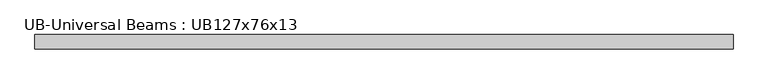
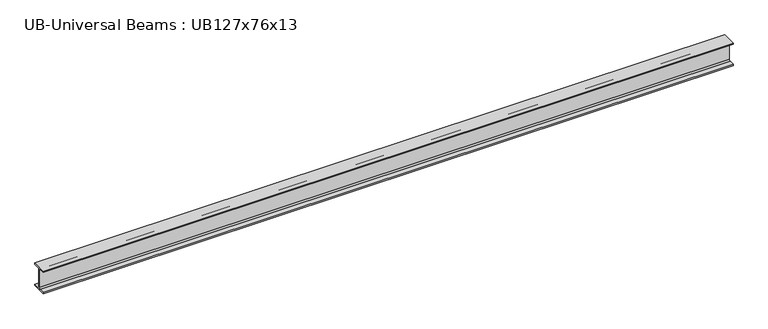
"""IFC4 building model written with IfcOpenShell, lengths in millimetres: member geometry, UB-Universal Beams : UB127x76x13."""

from ifc_helpers import new_model, si_unit, point, frame, frame_2d, origin, place, context, project, spatial, polyline, circle_curve, trimmed, segment, composite_curve, outline, extrude, source, transform, mapped, element, save


def ub_universal_beams_ub127x76x13_58dc6553(model_context):
    return source(origin(), model_context, "Body", "SweptSolid", [
        extrude(outline(composite_curve([segment(polyline([(38.0, -55.9), (38.0, -63.5), (-38.0, -63.5), (-38.0, -55.9), (-9.6, -55.9)]), True, "CONTINUOUS"), segment(trimmed(circle_curve(frame_2d((-9.6, -48.3)), 7.6), [point((-9.6, -55.9))], [point((-2.0, -48.3))], True, "CARTESIAN"), True, "CONTINUOUS"), segment(polyline([(-2.0, -48.3), (-2.0, 48.3)]), True, "CONTINUOUS"), segment(trimmed(circle_curve(frame_2d((-9.6, 48.3)), 7.6), [point((-2.0, 48.3))], [point((-9.6, 55.9))], True, "CARTESIAN"), True, "CONTINUOUS"), segment(polyline([(-9.6, 55.9), (-38.0, 55.9), (-38.0, 63.5), (38.0, 63.5), (38.0, 55.9), (9.6, 55.9)]), True, "CONTINUOUS"), segment(trimmed(circle_curve(frame_2d((9.6, 48.3)), 7.6), [point((9.6, 55.9))], [point((2.0, 48.3))], True, "CARTESIAN"), True, "CONTINUOUS"), segment(polyline([(2.0, 48.3), (2.0, -48.3)]), True, "CONTINUOUS"), segment(trimmed(circle_curve(frame_2d((9.6, -48.3)), 7.6), [point((2.0, -48.3))], [point((9.6, -55.9))], True, "CARTESIAN"), True, "CONTINUOUS"), segment(polyline([(9.6, -55.9), (38.0, -55.9)]), True, "CONTINUOUS")], self_intersect=False)), frame((-2049.1, 0.0, 0.0), z_axis=(1.0, 0.0, 0.0), x_axis=(0.0, 1.0, 0.0)), (0.0, 0.0, 1.0), 3676.2),
    ])


if __name__ == "__main__":
    model = new_model("IFC4")
    model_context = context("Model", 3, world=origin())
    ifc_project = project(units=[si_unit("LENGTHUNIT", "METRE", prefix="MILLI")], contexts=[model_context])
    site = spatial("IfcSite", under=ifc_project)
    building = spatial("IfcBuilding", under=site)
    placement = place(None, origin())
    ub_universal_beams_ub127x76x13_shape = ub_universal_beams_ub127x76x13_58dc6553(model_context)
    element("IfcMember", 1, ObjectType="UB-Universal Beams : UB127x76x13", at=placement, inside=building, context=model_context, shape_type="MappedRepresentation", body=[
        mapped(ub_universal_beams_ub127x76x13_shape, transform((0.0, 0.0, 0.0), x_axis=(1.0, 0.0, 0.0), y_axis=(0.0, 1.0, 0.0), z_axis=(0.0, 0.0, 1.0))),
    ])
    save(model, "model.ifc")

# Revit data of these elements
# Type "UB-Universal Beams : UB127x76x13"
#   Section Name Key = "UB127X76X13"
#   Width = 7.6 cm
#   Web Thickness = 0.4 cm
#   Web Fillet = 0.76 cm
#   Warping Constant = 2000.0 cm⁶
#   Torsional Moment of Inertia = 2.85 cm⁴
#   Section Area = 16.5 cm²
#   Plastic Modulus weak axis = 22.6 cm³
#   Plastic Modulus strong axis = 84.2 cm³
#   Nominal Weight = 13.00 kgf/m
#   Moment of Inertia weak axis = 55.70 cm⁴
#   Moment of Inertia strong axis = 473.00 cm⁴
#   Height = 12.7 cm
#   Flange Thickness = 0.76 cm
#   Elastic Modulus weak axis = 14.7 cm³
#   Elastic Modulus strong axis = 74.6 cm³
#   Centroid Vertical = 6.35 cm
#   Centroid Horizontal = 3.8 cm
#   Bolt Spacing = 4.0 cm
#   Length [instance default] = 1.5 m
#   Structural Material [instance default] = Metal - Steel 43-275
#   Type Comments = ""
#   Assembly Code = ""
# Element 1 (IfcMember, "UB-Universal Beams : UB127x76x13")
#   Materials on its faces: "Metal - Steel 43-275"
# Materials
#   "Metal - Steel 43-275": class "Metal", colour RGB 247 247 247, transparency 0, Cost = 0
